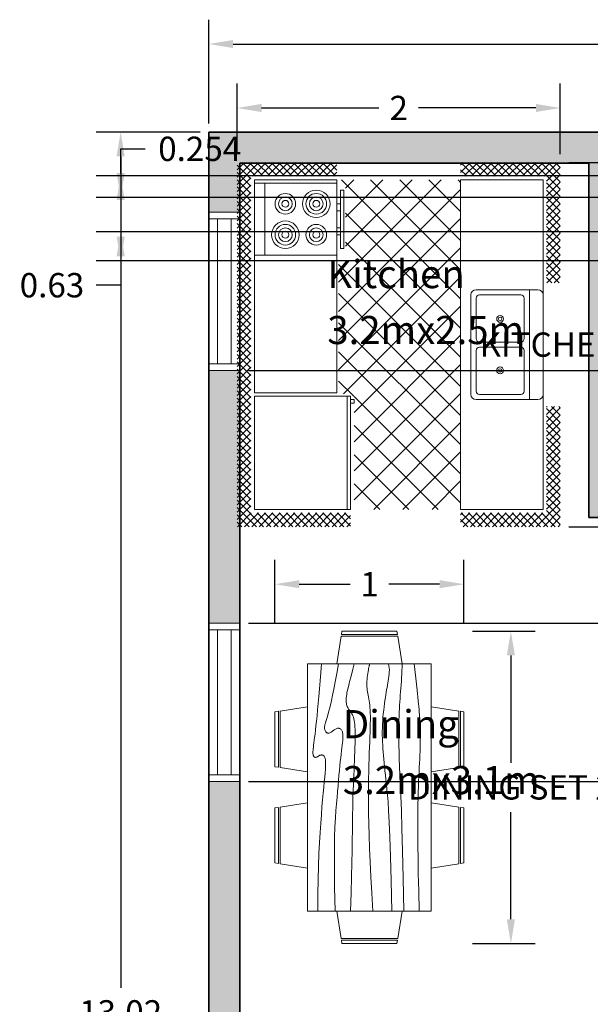
# Model space of a CAD drawing. Units: metres. Extents: x 35.2 to 46.4, y 446.1 to 460.8.
# Tile 5 of 6: x 36.2 to 40.4, y 453.5 to 460.8. Entities that reach past the tile are written whole.
import ezdxf

# ---------------------------------------------------------------- set-up
doc = ezdxf.new("R2010")
doc.units = ezdxf.units.M
for name, color, linetype, lineweight in [('A-ANNO-DIMS', 2, 'Continuous', 18), ('A-AREA-IDEN', 7, 'Continuous', 18), ('A-FLOR-FIXT', 9, 'Continuous', 18), ('A-GLAZ', 4, 'Continuous', 18), ('A-WALL', 7, 'Continuous', 35), ('A-WALL-PATT', 252, 'Continuous', 13), ('FURNITURE', 53, 'Continuous', 18)]:
    doc.layers.add(name, color=color, linetype=linetype, lineweight=lineweight)
doc.styles.get("Standard").update_dxf_attribs({"font": 'calibri.ttf'})
doc.dimstyles.get("Standard").update_dxf_attribs({"dimtxt": 0.18, "dimasz": 0.18, "dimexe": 0.18, "dimexo": 0.0625, "dimgap": 0.09, "dimtad": 0, "dimtih": 1, "dimtoh": 1, "dimdec": 4, "dimzin": 0, "dimdsep": 46, "dimtxsty": 'Standard', "dimcen": 0.09, "dimadec": 0, "dimazin": 0, "dimtfac": 1, "dimtdec": 4, "dimtofl": 0, "dimtmove": 0, "dimatfit": 3, "dimfxl": 1, "dimtolj": 1, "dimtzin": 0, "dimarcsym": 0})

# ---------------------------------------------------------------- blocks, each defined once
blk = doc.blocks.new('Dining Set - 36 x 72 in.')
for p, q in [((-22.2343, 26.00059), (-23.4847, 17.99762)), ((-22.2304, 26), (-5.7608, 26)), ((-22, 27.5), (-22.1562, 26.50042)), ((-5.8416, 26.5), (-22.1534, 26.5)), ((-22, 27.5), (-6, 27.5)), ((-5.8437, 26.49966), (-6, 27.5)), ((-4.5152, 17.99762), (-5.7655, 25.99926)), ((5.7657, 26.00059), (4.5153, 17.99762)), ((5.7696, 26), (22.2392, 26)), ((6, 27.5), (5.8438, 26.50042)), ((22.1584, 26.5), (5.8466, 26.5)), ((6, 27.5), (22, 27.5)), ((22.1563, 26.49966), (22, 27.5)), ((23.4848, 17.99762), (22.2345, 25.99926)), ((36, 18), (-36, 18)), ((-36, 18), (-36, -18)), ((36, -18), (36, 18)), ((-44.0006, 8.23428), (-35.9976, 9.48474)), ((44.0006, 8.23428), (35.9976, 9.48474)), ((-45.5, 8), (-44.5004, 8.15617)), ((-45.5, 8), (-45.5, -8)), ((-44.5, -8.15843), (-44.5, 8.15338)), ((-44, 8.23041), (-44, -8.23915)), ((44, 8.23041), (44, -8.23915)), ((44.5, -8.15843), (44.5, 8.15338)), ((45.5, 8), (44.5005, 8.15617)), ((45.5, 8), (45.5, -8)), ((-44.4997, -8.15631), (-45.5, -8)), ((-35.9976, -9.48476), (-43.9993, -8.2345)), ((35.9976, -9.48476), (43.9993, -8.2345)), ((44.4997, -8.15631), (45.5, -8)), ((-36, -18), (36, -18)), ((-22.2343, -26.0006), (-23.4847, -17.99762)), ((-4.5152, -17.99762), (-5.7655, -25.99928)), ((5.7657, -26.0006), (4.5153, -17.99762)), ((23.4848, -17.99762), (22.2345, -25.99928)), ((-22.2304, -26), (-5.7608, -26)), ((-22, -27.5), (-22.1562, -26.50044)), ((-5.8416, -26.5), (-22.1534, -26.5)), ((-22, -27.5), (-6, -27.5)), ((-5.8437, -26.49967), (-6, -27.5)), ((5.7696, -26), (22.2392, -26)), ((6, -27.5), (5.8438, -26.50044)), ((22.1584, -26.5), (5.8466, -26.5)), ((6, -27.5), (22, -27.5)), ((22.1563, -26.49967), (22, -27.5))]:
    blk.add_line(p, q)
for points in [[(-36, 15), (-31.1772, 14.97754), (-26.8079, 14.91406), (-22.8538, 14.81543), (-19.276, 14.6875), (-16.0362, 14.53613), (-13.0957, 14.36718), (-10.4159, 14.18652), (-7.9583, 14), (-5.6904, 13.81315), (-3.6035, 13.63021), (-1.6954, 13.45508), (0.0365, 13.29166), (1.5945, 13.14388), (2.9811, 13.01562), (4.1988, 12.9108), (5.25, 12.83333), (6.1393, 12.78613), (6.8802, 12.76823), (7.4883, 12.77767), (7.9792, 12.8125), (8.3685, 12.87077), (8.6719, 12.95052), (8.9049, 13.0498), (9.0833, 13.16666), (9.2205, 13.29899), (9.3216, 13.44401), (9.3895, 13.59879), (9.4271, 13.76041), (9.4373, 13.92594), (9.4232, 14.09245), (9.3875, 14.257), (9.3333, 14.41666), (9.2638, 14.56917), (9.1836, 14.71484), (9.0975, 14.85465), (9.0104, 14.98958), (8.9272, 15.1206), (8.8529, 15.2487), (8.7922, 15.37483), (8.75, 15.5), (8.7305, 15.62467), (8.7344, 15.74739), (8.7617, 15.86621), (8.8125, 15.97916), (8.8867, 16.08431), (8.9844, 16.17968), (9.1055, 16.26334), (9.25, 16.33333), (9.4189, 16.38802), (9.6172, 16.42708), (9.8506, 16.45052), (10.125, 16.45833), (10.4463, 16.45052), (10.8203, 16.42708), (11.2529, 16.38802), (11.75, 16.33333), (12.3184, 16.26318), (12.9694, 16.17838), (13.7151, 16.07991), (14.5677, 15.96875), (15.5395, 15.84586), (16.6426, 15.71224), (17.8893, 15.56884), (19.2917, 15.41666), (20.859, 15.25667), (22.5879, 15.08984), (24.4721, 14.91715), (26.5052, 14.73958), (28.6809, 14.5581), (30.9929, 14.3737), (33.4347, 14.18733), (36, 14)], [(-36, 10), (-28.9766, 10.14274), (-23.1725, 10.20442), (-18.4241, 10.19775), (-14.5677, 10.13541), (-11.4399, 10.03011), (-8.877, 9.89453), (-6.7154, 9.74137), (-4.7917, 9.58333), (-2.9698, 9.43082), (-1.2246, 9.28515), (0.4415, 9.14534), (2.026, 9.01041), (3.5266, 8.87939), (4.9408, 8.7513), (6.266, 8.62516), (7.5, 8.5), (8.6411, 8.37549), (9.6914, 8.2539), (10.6538, 8.13818), (11.5312, 8.03125), (12.3267, 7.93603), (13.043, 7.85547), (13.6831, 7.79248), (14.25, 7.75), (14.7471, 7.7303), (15.1797, 7.73307), (15.5537, 7.75732), (15.875, 7.80208), (16.1494, 7.86637), (16.3828, 7.94922), (16.5811, 8.04964), (16.75, 8.16666), (16.8944, 8.29915), (17.0143, 8.44531), (17.1089, 8.60319), (17.1771, 8.77083), (17.218, 8.94629), (17.2305, 9.1276), (17.2137, 9.31282), (17.1667, 9.5), (17.0895, 9.6875), (16.987, 9.875), (16.8649, 10.0625), (16.7292, 10.25), (16.5856, 10.4375), (16.4401, 10.625), (16.2985, 10.8125), (16.1667, 11), (16.05, 11.18733), (15.9518, 11.3737), (15.8752, 11.5581), (15.8229, 11.73958), (15.798, 11.91715), (15.8034, 12.08984), (15.842, 12.25667), (15.9167, 12.41666), (16.0295, 12.56836), (16.1784, 12.70833), (16.3605, 12.83268), (16.5729, 12.9375), (16.8127, 13.01888), (17.0768, 13.07291), (17.3625, 13.0957), (17.6667, 13.08333), (17.9894, 13.03312), (18.3418, 12.94726), (18.7382, 12.82918), (19.1927, 12.68229), (19.7195, 12.51001), (20.3327, 12.31575), (21.0465, 12.10294), (21.875, 11.875), (22.8357, 11.63354), (23.959, 11.37304), (25.2786, 11.08618), (26.8282, 10.76562), (28.6414, 10.40405), (30.752, 9.99414), (33.1936, 9.52856), (36, 9)], [(-36, 5.5), (-30.7157, 5.3348), (-26.069, 5.20963), (-21.9946, 5.11767), (-18.4271, 5.05208), (-15.3009, 5.00602), (-12.5508, 4.97265), (-10.1112, 4.94515), (-7.9167, 4.91666), (-5.909, 4.88167), (-4.0586, 4.83984), (-2.3429, 4.79215), (-0.7396, 4.73958), (0.7739, 4.6831), (2.22, 4.6237), (3.6213, 4.56233), (5, 4.5), (6.373, 4.43782), (7.7344, 4.3776), (9.0723, 4.32129), (10.375, 4.27083), (11.6309, 4.22819), (12.8281, 4.19531), (13.9551, 4.17415), (15, 4.16666), (15.954, 4.17448), (16.819, 4.19791), (17.6001, 4.23698), (18.3021, 4.29166), (18.9299, 4.36198), (19.4883, 4.44791), (19.9823, 4.54948), (20.4167, 4.66666), (20.7969, 4.79899), (21.1302, 4.94401), (21.4245, 5.09879), (21.6875, 5.26041), (21.9271, 5.42594), (22.1511, 5.59245), (22.3672, 5.757), (22.5834, 5.91666), (22.8065, 6.06868), (23.0404, 6.21093), (23.2879, 6.34147), (23.5521, 6.45833), (23.8358, 6.55957), (24.142, 6.64323), (24.4735, 6.70735), (24.8334, 6.75), (25.2235, 6.76969), (25.642, 6.76692), (26.0858, 6.74267), (26.5521, 6.69791), (27.0379, 6.63362), (27.5404, 6.55078), (28.0565, 6.45036), (28.5834, 6.33333), (29.1242, 6.19987), (29.7071, 6.04687), (30.3661, 5.87044), (31.1354, 5.66666), (32.0493, 5.43164), (33.142, 5.16146), (34.4475, 4.85221), (36, 4.5)], [(-36, -1), (-30.7915, -0.6591), (-26.0195, -0.38216), (-21.6519, -0.16284), (-17.6563, 0.00521), (-14.0005, 0.12833), (-10.6523, 0.21289), (-7.5796, 0.26522), (-4.75, 0.29166), (-2.134, 0.29793), (0.2878, 0.28711), (2.5317, 0.26163), (4.6146, 0.22396), (6.5529, 0.17651), (8.3633, 0.12174), (10.0623, 0.06209), (11.6667, 0), (13.1899, -0.06201), (14.6341, -0.1211), (15.9982, -0.17432), (17.2813, -0.21875), (18.4823, -0.25147), (19.6003, -0.26953), (20.6343, -0.27002), (21.5834, -0.25), (22.4481, -0.20768), (23.2357, -0.14584), (23.9549, -0.06836), (24.6146, 0.02083), (25.2235, 0.11784), (25.7904, 0.21875), (26.3241, 0.31966), (26.8334, 0.41666), (27.3265, 0.50618), (27.8099, 0.58593), (28.2894, 0.65397), (28.7709, 0.70833), (29.2601, 0.74707), (29.763, 0.76823), (30.2855, 0.76985), (30.8334, 0.75), (31.4088, 0.70784), (31.9994, 0.64713), (32.589, 0.57275), (33.1615, 0.48958), (33.7008, 0.4025), (34.1908, 0.3164), (34.6153, 0.23616), (34.9584, 0.16666), (35.2099, 0.11165), (35.3848, 0.07031), (35.504, 0.04069), (35.5886, 0.02083), (35.6594, 0.00879), (35.7377, 0.0026), (35.8442, 0.00032), (36, 0)], [(-36, -6.5), (-27.1843, -6.31267), (-20.084, -6.1263), (-14.469, -5.9419), (-10.1094, -5.76042), (-6.7752, -5.58285), (-4.2363, -5.41016), (-2.2629, -5.24333), (-0.625, -5.08334), (0.8708, -4.93099), (2.2715, -4.78646), (3.5872, -4.64974), (4.8281, -4.52084), (6.0046, -4.39974), (7.127, -4.28646), (8.2053, -4.18099), (9.25, -4.08334), (10.2705, -3.99382), (11.2734, -3.91407), (12.2647, -3.84603), (13.25, -3.79167), (14.2354, -3.75293), (15.2266, -3.73177), (16.2295, -3.73015), (17.25, -3.75), (18.2912, -3.79248), (19.3451, -3.85547), (20.4009, -3.93604), (21.4479, -4.03125), (22.4754, -4.13819), (23.4727, -4.25391), (24.4289, -4.37549), (25.3334, -4.5), (26.1785, -4.62492), (26.9694, -4.74935), (27.7145, -4.87281), (28.4219, -4.99479), (29.1, -5.11483), (29.7572, -5.23242), (30.4016, -5.34709), (31.0417, -5.45834), (31.6837, -5.56437), (32.3262, -5.65821), (32.9658, -5.73153), (33.599, -5.77604), (34.2224, -5.78345), (34.8327, -5.74545), (35.4264, -5.65373), (36, -5.5)], [(-36, -10), (-26.4022, -9.81299), (-18.4675, -9.62891), (-11.9839, -9.45069), (-6.7396, -9.28125), (-2.5226, -9.12354), (0.8789, -8.98047), (3.6769, -8.85498), (6.0833, -8.75), (8.2767, -8.66765), (10.3021, -8.60677), (12.1712, -8.56543), (13.8958, -8.54167), (15.4876, -8.53353), (16.9583, -8.53907), (18.3197, -8.55632), (19.5834, -8.58334), (20.7616, -8.61841), (21.8685, -8.66081), (22.9188, -8.71004), (23.9271, -8.76563), (24.9081, -8.82707), (25.8763, -8.89388), (26.8465, -8.96558), (27.8334, -9.04167), (28.8474, -9.12118), (29.8828, -9.20117), (30.93, -9.27824), (31.9792, -9.34896), (33.0205, -9.40991), (34.0443, -9.45768), (35.0407, -9.48885), (36, -9.5)], [(-36, -14.5), (-30.0881, -14.33513), (-25.0332, -14.21224), (-20.7312, -14.12647), (-17.0781, -14.07292), (-13.97, -14.04671), (-11.3027, -14.04297), (-8.9724, -14.05681), (-6.875, -14.08334), (-4.9224, -14.11833), (-3.0905, -14.16016), (-1.3709, -14.20785), (0.2448, -14.26042), (1.7647, -14.3169), (3.1973, -14.3763), (4.5507, -14.43767), (5.8333, -14.5), (7.0554, -14.5621), (8.235, -14.62175), (9.3922, -14.67652), (10.5469, -14.72396), (11.7192, -14.76164), (12.929, -14.78711), (14.1965, -14.79794), (15.5417, -14.79167), (16.9933, -14.76424), (18.6152, -14.70508), (20.4804, -14.60197), (22.6615, -14.44271), (25.2312, -14.21509), (28.2624, -13.9069), (31.8277, -13.50594), (36, -13)]]:
    blk.add_lwpolyline(points)
blk = doc.blocks.new('Kitchen Layout - 7 x 8 ft')
for p, q in [((-5, 81.32), (2.68, 89)), ((-5, 83.44), (0.56, 89)), ((-5, 85.56), (-1.56, 89)), ((-5, 87.68), (-3.68, 89)), ((-1, 84.97), (-5, 88.97)), ((1.09, 85), (-2.91, 89)), ((3.21, 85), (-0.79, 89)), ((0.81, 85), (4.81, 89)), ((5.34, 85), (1.34, 89)), ((2.93, 85), (6.93, 89)), ((7.46, 85), (3.46, 89)), ((5.05, 85), (9.05, 89)), ((9.58, 85), (5.58, 89)), ((7.17, 85), (11.17, 89)), ((11.7, 85), (7.7, 89)), ((9.29, 85), (13.29, 89)), ((13.82, 85), (9.82, 89)), ((11.41, 85), (15.41, 89)), ((15.94, 85), (11.94, 89)), ((13.53, 85), (17.53, 89)), ((18.06, 85), (14.06, 89)), ((15.65, 85), (19.65, 89)), ((20.18, 85), (16.18, 89)), ((17.78, 85), (21.78, 89)), ((22.31, 85), (18.31, 89)), ((19.9, 85), (23.9, 89)), ((24.43, 85), (20.43, 89)), ((22.02, 85), (26.02, 89)), ((26.55, 85), (22.55, 89)), ((24.14, 85), (28.14, 89)), ((28.67, 85), (24.67, 89)), ((26.26, 85), (30.26, 89)), ((30.79, 85), (26.79, 89)), ((28.38, 85), (32.38, 89)), ((32.91, 85), (28.91, 89)), ((30.5, 85), (34.5, 89)), ((35.03, 85), (31.03, 89)), ((32.63, 85), (36.63, 89)), ((37.16, 85), (33.16, 89)), ((34.75, 85), (38.75, 89)), ((39.28, 85), (35.28, 89)), ((36.87, 85), (40.87, 89)), ((41.4, 85), (37.4, 89)), ((38.99, 85), (42.99, 89)), ((43.52, 85), (39.52, 89)), ((41.11, 85), (45.11, 89)), ((45.64, 85), (41.64, 89)), ((43.23, 85), (47.23, 89)), ((47.76, 85), (43.76, 89)), ((45.35, 85), (49.35, 89)), ((49.88, 85), (45.88, 89)), ((47.47, 85), (51.47, 89)), ((52, 85), (48, 89)), ((49.6, 85), (53.6, 89)), ((54.13, 85), (50.13, 89)), ((51.72, 85), (55.72, 89)), ((56.25, 85), (52.25, 89)), ((53.84, 85), (57.84, 89)), ((58.37, 85), (54.37, 89)), ((55.96, 85), (59.96, 89)), ((60.49, 85), (56.49, 89)), ((58.08, 85), (62.08, 89)), ((62.61, 85), (58.61, 89)), ((60.2, 85), (64.2, 89)), ((64.73, 85), (60.73, 89)), ((62.32, 85), (66.32, 89)), ((66.85, 85), (62.85, 89)), ((64.45, 85), (68.45, 89)), ((68.97, 85), (64.97, 89)), ((66.57, 85), (70.57, 89)), ((71.1, 85), (67.1, 89)), ((68.69, 85), (72.69, 89)), ((73.22, 85), (69.22, 89)), ((70.81, 85), (74.81, 89)), ((75.34, 85), (71.34, 89)), ((72.93, 85), (76.93, 89)), ((77.46, 85), (73.46, 89)), ((75.05, 85), (79.05, 89)), ((79.58, 85), (75.58, 89)), ((77.17, 85), (81.17, 89)), ((81.7, 85), (77.7, 89)), ((79.29, 85), (83.29, 89)), ((83.82, 85), (79.82, 89)), ((81.42, 85), (85.42, 89)), ((85.95, 85), (81.95, 89)), ((83.54, 85), (87.54, 89)), ((88.07, 85), (84.07, 89)), ((85.66, 85), (89.66, 89)), ((90.19, 85), (86.19, 89)), ((87.78, 85), (91.78, 89)), ((92.31, 85), (88.31, 89)), ((89.9, 85), (93.9, 89)), ((94.43, 85), (90.43, 89)), ((92.02, 85), (96.02, 89)), ((96.55, 85), (92.55, 89)), ((94.14, 85), (98.14, 89)), ((101, 82.67), (94.67, 89)), ((96.27, 85), (100.27, 89)), ((101, 84.79), (96.79, 89)), ((101, 86.92), (98.92, 89)), ((-1, 82.85), (-5, 86.85)), ((97, 83.61), (101, 87.61)), ((-1, 80.73), (-5, 84.73)), ((-5, 79.19), (-1, 83.19)), ((34, 84), (96, 84)), ((34, 60), (34, 84)), ((96, 84), (96, 60)), ((97, 81.49), (101, 85.49)), ((101, 80.55), (97, 84.55)), ((97, 79.37), (101, 83.37)), ((-1, 78.61), (-5, 82.61)), ((-5, 77.07), (-1, 81.07)), ((-1, 76.49), (-5, 80.49)), ((74, 81), (95, 81)), ((101, 78.43), (97, 82.43)), ((97, 77.25), (101, 81.25)), ((101, 76.31), (97, 80.31)), ((-5, 74.95), (-1, 78.95)), ((-1, 74.36), (-5, 78.36)), ((97, 75.13), (101, 79.13)), ((101, 74.19), (97, 78.19)), ((-5, 72.83), (-1, 76.83)), ((-1, 72.24), (-5, 76.24)), ((-5, 70.71), (-1, 74.71)), ((97, 73.01), (101, 77.01)), ((101, 72.07), (97, 76.07)), ((97, 70.89), (101, 74.89)), ((-1, 70.12), (-5, 74.12)), ((-5, 68.59), (-1, 72.59)), ((-1, 68), (-5, 72)), ((101, 69.95), (97, 73.95)), ((97, 68.76), (101, 72.76)), ((101, 67.82), (97, 71.82)), ((-5, 66.47), (-1, 70.47)), ((-1, 65.88), (-5, 69.88)), ((97, 66.64), (101, 70.64)), ((101, 65.7), (97, 69.7)), ((-5, 64.35), (-1, 68.35)), ((-1, 63.76), (-5, 67.76)), ((-5, 62.22), (-1, 66.22)), ((97, 64.52), (101, 68.52)), ((101, 63.58), (97, 67.58)), ((97, 62.4), (101, 66.4)), ((-1, 61.64), (-5, 65.64)), ((-5, 60.1), (-1, 64.1)), ((-1, 59.52), (-5, 63.52)), ((101, 61.46), (97, 65.46)), ((97, 60.28), (101, 64.28)), ((100.34, 60), (97, 63.34)), ((-5, 57.98), (-1, 61.98)), ((-1, 57.39), (-5, 61.39)), ((98.22, 60), (97, 61.22)), ((98.84, 60), (101, 62.16)), ((-1.73, 56), (-5, 59.27)), ((-4.86, 56), (-1, 59.86)), ((-2.74, 56), (-1, 57.74)), ((10.4, 24), (45.9, 59.5)), ((18.88, 24), (54.38, 59.5)), ((27.37, 24), (62.87, 59.5)), ((33.03, 55.11), (37.41, 59.5)), ((67.71, 24), (33.68, 58.04)), ((96, 60), (34, 60)), ((35.85, 24), (71.35, 59.5)), ((76.2, 24), (40.7, 59.5)), ((44.34, 24), (77.84, 57.5)), ((84.68, 24), (49.18, 59.5)), ((52.82, 24), (86.32, 57.5)), ((93.17, 24), (57.67, 59.5)), ((61.31, 24), (96, 58.69)), ((96, 29.65), (66.15, 59.5)), ((96, 38.14), (76.64, 57.5)), ((80, 60), (80, 59)), ((82, 59), (82, 60)), ((96, 46.63), (85.13, 57.5)), ((87, 59), (87, 60)), ((89, 60), (89, 59)), ((96, 55.11), (93.57, 57.54)), ((100.96, 60), (101, 60.04)), ((-3.85, 56), (-5, 57.15)), ((0, 57), (33, 57)), ((0, 30.57), (24.43, 55)), ((0, 39.06), (15.94, 55)), ((0, 47.54), (7.46, 55)), ((1.91, 24), (32.91, 55)), ((33.77, 24), (2.77, 55)), ((42.26, 24), (11.26, 55)), ((50.74, 24), (19.74, 55)), ((59.23, 24), (28.23, 55)), ((31, 55), (31, 56)), ((32, 55), (31, 55)), ((32, 56), (32, 55)), ((25.29, 24), (0, 49.29)), ((69.79, 24), (96, 50.21)), ((16.8, 24), (0, 40.8)), ((78.28, 24), (96, 41.72)), ((8.32, 24), (0, 32.32)), ((86.76, 24), (96, 33.24)), ((-5, 21.92), (-2.92, 24)), ((-5, 19.8), (-1, 23.8)), ((-1, 19.21), (-5, 23.21)), ((-1, 21.33), (-3.67, 24)), ((-1, 23.45), (-1.55, 24)), ((0, 24), (96, 24)), ((0, 0), (0, 24)), ((95.25, 24), (96, 24.75)), ((96, 24), (96, 0)), ((97, 22.1), (98.9, 24)), ((97, 19.97), (101, 23.97)), ((101, 19.03), (97, 23.03)), ((101, 21.16), (98.16, 24)), ((101, 23.28), (100.28, 24)), ((-5, 17.68), (-1, 21.68)), ((-1, 17.09), (-5, 21.09)), ((97, 17.85), (101, 21.85)), ((101, 16.91), (97, 20.91)), ((-5, 15.55), (-1, 19.55)), ((-1, 14.97), (-5, 18.97)), ((-5, 13.43), (-1, 17.43)), ((47.25, 6.5), (47.25, 18.5)), ((48.75, 18.5), (48.75, 6.5)), ((97, 15.73), (101, 19.73)), ((101, 14.79), (97, 18.79)), ((97, 13.61), (101, 17.61)), ((-1, 12.85), (-5, 16.85)), ((-5, 11.31), (-1, 15.31)), ((-1, 10.73), (-5, 14.73)), ((101, 12.67), (97, 16.67)), ((97, 11.49), (101, 15.49)), ((101, 10.55), (97, 14.55)), ((-5, 9.19), (-1, 13.19)), ((-1, 8.6), (-5, 12.6)), ((97, 9.37), (101, 13.37)), ((101, 8.43), (97, 12.43)), ((-5, 7.07), (-1, 11.07)), ((-1, 6.48), (-5, 10.48)), ((-5, 4.95), (-1, 8.95)), ((97, 7.25), (101, 11.25)), ((101, 6.31), (97, 10.31)), ((97, 5.12), (101, 9.12)), ((-1, 4.36), (-5, 8.36)), ((-5, 2.83), (-1, 6.83)), ((-1, 2.24), (-5, 6.24)), ((101, 4.18), (97, 8.18)), ((97, 3), (101, 7)), ((101, 2.06), (97, 6.06)), ((-5, 0.71), (-1, 4.71)), ((-1, 0.12), (-5, 4.12)), ((64, 4), (32, 4)), ((97, 0.88), (101, 4.88)), ((101, -0.06), (97, 3.94)), ((-5, -1.42), (-1, 2.58)), ((2, -5), (-5, 2)), ((-5, -3.54), (-1, 0.46)), ((96, 0), (0, 0)), ((93.24, -5), (101, 2.76)), ((95.36, -5), (101, 0.64)), ((101, -2.18), (97, 1.82)), ((-0.12, -5), (-5, -0.12)), ((-2.25, -5), (-5, -2.25)), ((-4.34, -5), (-0.34, -1)), ((-2.22, -5), (1.78, -1)), ((-0.1, -5), (3.9, -1)), ((4.12, -5), (0.12, -1)), ((2.02, -5), (6.02, -1)), ((6.24, -5), (2.24, -1)), ((4.14, -5), (8.14, -1)), ((8.36, -5), (4.36, -1)), ((6.27, -5), (10.27, -1)), ((10.48, -5), (6.48, -1)), ((8.39, -5), (12.39, -1)), ((12.6, -5), (8.6, -1)), ((10.51, -5), (14.51, -1)), ((14.73, -5), (10.73, -1)), ((12.63, -5), (16.63, -1)), ((16.85, -5), (12.85, -1)), ((14.75, -5), (18.75, -1)), ((18.97, -5), (14.97, -1)), ((16.87, -5), (20.87, -1)), ((21.09, -5), (17.09, -1)), ((18.99, -5), (22.99, -1)), ((23.21, -5), (19.21, -1)), ((21.11, -5), (25.11, -1)), ((25.33, -5), (21.33, -1)), ((23.24, -5), (27.24, -1)), ((27.45, -5), (23.45, -1)), ((25.36, -5), (29.36, -1)), ((29.57, -5), (25.57, -1)), ((27.48, -5), (30, -2.48)), ((30, -3.3), (27.7, -1)), ((30, -1.18), (29.82, -1)), ((66, -2.54), (67.54, -1)), ((66, -4.66), (69.66, -1)), ((69.88, -5), (66, -1.12)), ((67.78, -5), (71.78, -1)), ((72, -5), (68, -1)), ((69.9, -5), (73.9, -1)), ((74.12, -5), (70.12, -1)), ((72.03, -5), (76.03, -1)), ((76.24, -5), (72.24, -1)), ((74.15, -5), (78.15, -1)), ((78.36, -5), (74.36, -1)), ((76.27, -5), (80.27, -1)), ((80.49, -5), (76.49, -1)), ((78.39, -5), (82.39, -1)), ((82.61, -5), (78.61, -1)), ((80.51, -5), (84.51, -1)), ((84.73, -5), (80.73, -1)), ((82.63, -5), (86.63, -1)), ((86.85, -5), (82.85, -1)), ((84.75, -5), (88.75, -1)), ((88.97, -5), (84.97, -1)), ((86.88, -5), (90.88, -1)), ((91.09, -5), (87.09, -1)), ((89, -5), (93, -1)), ((93.21, -5), (89.21, -1)), ((91.12, -5), (95.12, -1)), ((95.34, -5), (91.34, -1)), ((97.46, -5), (93.46, -1)), ((99.58, -5), (95.58, -1)), ((101, -4.3), (97, -0.3)), ((97.48, -5), (101, -1.48)), ((-4.37, -5), (-5, -4.37)), ((29.6, -5), (30, -4.6)), ((67.76, -5), (66, -3.24)), ((99.6, -5), (101, -3.6))]:
    blk.add_line(p, q)
for points in [[(0, 56), (0, 84), (33, 84), (33, 56)], [(74, 60), (74, 84), (95, 84), (95, 60)], [(76, 58), (76, 59), (93, 59), (93, 58)]]:
    blk.add_lwpolyline(points, close=True)
for points in [[(33.5, 21), (62.5, 21)], [(32, 1.5), (32, 19.5)], [(33.5, 6.5), (33.5, 18.5)], [(34.5, 19.5), (46.25, 19.5)], [(49.75, 19.5), (61.5, 19.5)], [(62.5, 18.5), (62.5, 6.5)], [(64, 19.5), (64, 1.5)], [(46.25, 5.5), (34.5, 5.5)], [(61.5, 5.5), (49.75, 5.5)], [(62.5, 0), (33.5, 0)]]:
    blk.add_lwpolyline(points)
for centre, radius in [((80, 75), 4), ((80, 75), 3), ((89, 75), 3), ((80, 75), 2), ((80, 75), 1), ((89, 75), 2), ((89, 75), 1), ((80, 66), 3), ((89, 66), 4), ((89, 66), 3), ((80, 66), 2), ((80, 66), 1), ((89, 66), 2), ((89, 66), 1), ((40.5, 12.5), 1), ((40.5, 12.5), 0.5), ((55.5, 12.5), 1), ((55.5, 12.5), 0.5)]:
    blk.add_circle(centre, radius)
for centre, radius, start, end in [((33.5, 19.5), 1.5, 90, 180), ((62.5, 19.5), 1.5, 0, 90), ((34.5, 18.5), 1, 90, 180), ((46.25, 18.5), 1, 0, 90), ((49.75, 18.5), 1, 90, 180), ((61.5, 18.5), 1, 0, 90), ((34.5, 6.5), 1, 180, 270), ((46.25, 6.5), 1, 270, 0), ((49.75, 6.5), 1, 180, 270), ((61.5, 6.5), 1, 270, 0), ((33.5, 1.5), 1.5, 180, 270), ((62.5, 1.5), 1.5, 270, 0)]:
    blk.add_arc(centre, radius, start, end)
blk = doc.blocks.new('WIN-1172')
for p, q in [((0, 1.1716), (0.23, 1.1716)), ((0, 1.1716), (0, 0)), ((0.23, 1.1716), (0.23, 0)), ((0, 1.1216), (0.23, 1.1216)), ((0.065, 1.1216), (0.065, 0.05)), ((0.165, 1.1216), (0.165, 0.05)), ((0.23, 0.05), (0, 0.05)), ((0.23, 0), (0, 0))]:
    blk.add_line(p, q)
blk = doc.blocks.new('*D139')
at = {"layer": 'A-ANNO-DIMS', "color": 0, "lineweight": -2, "transparency": 16777216}
for p, q in [((39.5553, 456.2345), (40.0195, 456.2345)), ((39.8395, 456.0545), (39.8395, 455.261)), ((39.8395, 454.1031), (39.8395, 454.8966)), ((39.5553, 453.9231), (40.0195, 453.9231))]:
    blk.add_line(p, q, dxfattribs=at)
at = {"layer": 'A-ANNO-DIMS', "color": 0, "transparency": 16777216}
for points in [[(39.8095, 456.0545), (39.8695, 456.0545), (39.8395, 456.2345)], [(39.8095, 454.1031), (39.8695, 454.1031), (39.8395, 453.9231)]]:
    blk.add_solid(points, dxfattribs=at)
at = {"layer": 'Defpoints', "color": 0, "transparency": 16777216}
for p in [(39.4928, 456.2345), (39.8395, 456.2345), (39.4928, 453.9231)]:
    blk.add_point(p, dxfattribs=at)
at = {"layer": 'A-ANNO-DIMS', "color": 0, "transparency": 16777216, "insert": (39.8395, 455.0788), "char_height": 0.18, "attachment_point": 5}
blk.add_mtext('\\A1;DINING SET 2', dxfattribs=at)
blk = doc.blocks.new('*D140')
at = {"layer": 'A-ANNO-DIMS', "color": 0, "lineweight": -2, "transparency": 16777216}
for p, q in [((38.0958, 456.297), (38.0958, 456.7612)), ((39.4928, 456.297), (39.4928, 456.7612)), ((38.2758, 456.5812), (38.6522, 456.5812)), ((39.3128, 456.5812), (38.9364, 456.5812))]:
    blk.add_line(p, q, dxfattribs=at)
at = {"layer": 'A-ANNO-DIMS', "color": 0, "transparency": 16777216}
for points in [[(38.2758, 456.6112), (38.2758, 456.5512), (38.0958, 456.5812)], [(39.3128, 456.6112), (39.3128, 456.5512), (39.4928, 456.5812)]]:
    blk.add_solid(points, dxfattribs=at)
at = {"layer": 'Defpoints', "color": 0, "transparency": 16777216}
for p in [(38.0958, 456.5812), (38.0958, 456.2345), (39.4928, 456.2345)]:
    blk.add_point(p, dxfattribs=at)
at = {"layer": 'A-ANNO-DIMS', "color": 0, "transparency": 16777216, "insert": (38.7943, 456.5812), "char_height": 0.18, "attachment_point": 5}
blk.add_mtext('\\A1;1', dxfattribs=at)
blk = doc.blocks.new('*D145')
at = {"layer": 'A-ANNO-DIMS', "color": 0, "lineweight": -2, "transparency": 16777216}
for p, q in [((40.2671, 459.6992), (40.7885, 459.6992)), ((40.6085, 459.5192), (40.6085, 458.5353)), ((40.6085, 457.1868), (40.6085, 458.1708)), ((40.2671, 457.0068), (40.7885, 457.0068))]:
    blk.add_line(p, q, dxfattribs=at)
at = {"layer": 'A-ANNO-DIMS', "color": 0, "transparency": 16777216}
for points in [[(40.5785, 459.5192), (40.6385, 459.5192), (40.6085, 459.6992)], [(40.5785, 457.1868), (40.6385, 457.1868), (40.6085, 457.0068)]]:
    blk.add_solid(points, dxfattribs=at)
at = {"layer": 'Defpoints', "color": 0, "transparency": 16777216}
for p in [(40.2046, 459.6992), (40.6085, 459.6992), (40.2046, 457.0068)]:
    blk.add_point(p, dxfattribs=at)
at = {"layer": 'A-ANNO-DIMS', "color": 0, "transparency": 16777216, "insert": (40.6085, 458.353), "char_height": 0.18, "attachment_point": 5}
blk.add_mtext('\\A1;KITCHEN UNITS 3', dxfattribs=at)
blk = doc.blocks.new('*D146')
at = {"layer": 'A-ANNO-DIMS', "color": 0, "lineweight": -2, "transparency": 16777216}
for p, q in [((37.817, 459.7617), (37.817, 460.2831)), ((40.2046, 459.7617), (40.2046, 460.2831)), ((37.997, 460.1031), (38.8647, 460.1031)), ((40.0246, 460.1031), (39.1569, 460.1031))]:
    blk.add_line(p, q, dxfattribs=at)
at = {"layer": 'A-ANNO-DIMS', "color": 0, "transparency": 16777216}
for points in [[(37.997, 460.1331), (37.997, 460.0731), (37.817, 460.1031)], [(40.0246, 460.1331), (40.0246, 460.0731), (40.2046, 460.1031)]]:
    blk.add_solid(points, dxfattribs=at)
at = {"layer": 'Defpoints', "color": 0, "transparency": 16777216}
for p in [(37.817, 460.1031), (37.817, 459.6992), (40.2046, 459.6992)]:
    blk.add_point(p, dxfattribs=at)
at = {"layer": 'A-ANNO-DIMS', "color": 0, "transparency": 16777216, "insert": (39.0108, 460.1031), "char_height": 0.18, "attachment_point": 5}
blk.add_mtext('\\A1;2', dxfattribs=at)
blk = doc.blocks.new('*D151')
at = {"layer": 'A-ANNO-DIMS', "color": 0, "lineweight": -2, "transparency": 16777216}
for p, q in [((37.6066, 459.9873), (37.6066, 460.756)), ((44.9866, 459.9873), (44.9866, 460.756)), ((37.7866, 460.576), (40.9679, 460.576)), ((44.8066, 460.576), (41.6253, 460.576))]:
    blk.add_line(p, q, dxfattribs=at)
at = {"layer": 'A-ANNO-DIMS', "color": 0, "transparency": 16777216}
for points in [[(37.7866, 460.606), (37.7866, 460.546), (37.6066, 460.576)], [(44.8066, 460.606), (44.8066, 460.546), (44.9866, 460.576)]]:
    blk.add_solid(points, dxfattribs=at)
at = {"layer": 'Defpoints', "color": 0, "transparency": 16777216}
for p in [(44.9866, 460.576), (37.6066, 459.9248), (44.9866, 459.9248)]:
    blk.add_point(p, dxfattribs=at)
at = {"layer": 'A-ANNO-DIMS', "color": 0, "transparency": 16777216, "insert": (41.2966, 460.576), "char_height": 0.18, "attachment_point": 5}
blk.add_mtext('\\A1;7.38', dxfattribs=at)
blk = doc.blocks.new('*D152')
at = {"layer": 'A-ANNO-DIMS', "color": 0, "lineweight": -2, "transparency": 16777216}
for p, q in [((37.5441, 459.9248), (36.7754, 459.9248)), ((36.9554, 459.7448), (36.9554, 453.597)), ((36.9554, 447.0848), (36.9554, 453.2326)), ((37.5441, 446.9048), (36.7754, 446.9048))]:
    blk.add_line(p, q, dxfattribs=at)
at = {"layer": 'A-ANNO-DIMS', "color": 0, "transparency": 16777216}
for points in [[(36.9254, 459.7448), (36.9854, 459.7448), (36.9554, 459.9248)], [(36.9254, 447.0848), (36.9854, 447.0848), (36.9554, 446.9048)]]:
    blk.add_solid(points, dxfattribs=at)
at = {"layer": 'Defpoints', "color": 0, "transparency": 16777216}
for p in [(36.9554, 459.9248), (37.6066, 459.9248), (37.6066, 446.9048)]:
    blk.add_point(p, dxfattribs=at)
at = {"layer": 'A-ANNO-DIMS', "color": 0, "transparency": 16777216, "insert": (36.9554, 453.4148), "char_height": 0.18, "attachment_point": 5}
blk.add_mtext('\\A1;13.02', dxfattribs=at)
blk = doc.blocks.new('*D156')
at = {"layer": 'A-ANNO-DIMS', "color": 0, "lineweight": -2, "transparency": 16777216}
for p, q in [((37.8991, 455.122), (45.8178, 455.122)), ((45.6378, 454.942), (45.6378, 454.1543)), ((45.6378, 453.0022), (45.6378, 453.7898)), ((37.8991, 452.8222), (45.8178, 452.8222))]:
    blk.add_line(p, q, dxfattribs=at)
at = {"layer": 'A-ANNO-DIMS', "color": 0, "transparency": 16777216}
for points in [[(45.6078, 454.942), (45.6678, 454.942), (45.6378, 455.122)], [(45.6078, 453.0022), (45.6678, 453.0022), (45.6378, 452.8222)]]:
    blk.add_solid(points, dxfattribs=at)
at = {"layer": 'Defpoints', "color": 0, "transparency": 16777216}
for p in [(37.8366, 455.122), (45.6378, 455.122), (37.8366, 452.8222)]:
    blk.add_point(p, dxfattribs=at)
at = {"layer": 'A-ANNO-DIMS', "color": 0, "transparency": 16777216, "insert": (45.6378, 453.9721), "char_height": 0.18, "attachment_point": 5}
blk.add_mtext('\\A1;2.3', dxfattribs=at)
blk = doc.blocks.new('*D157')
at = {"layer": 'A-ANNO-DIMS', "color": 0, "lineweight": -2, "transparency": 16777216}
for p, q in [((37.8991, 456.2935), (45.8178, 456.2935)), ((45.6378, 456.1135), (45.6378, 455.8886)), ((45.6378, 455.302), (45.6378, 455.5269)), ((37.8991, 455.122), (45.8178, 455.122))]:
    blk.add_line(p, q, dxfattribs=at)
at = {"layer": 'A-ANNO-DIMS', "color": 0, "transparency": 16777216}
for points in [[(45.6078, 456.1135), (45.6678, 456.1135), (45.6378, 456.2935)], [(45.6078, 455.302), (45.6678, 455.302), (45.6378, 455.122)]]:
    blk.add_solid(points, dxfattribs=at)
at = {"layer": 'Defpoints', "color": 0, "transparency": 16777216}
for p in [(37.8366, 456.2935), (45.6378, 456.2935), (37.8366, 455.122)]:
    blk.add_point(p, dxfattribs=at)
at = {"layer": 'A-ANNO-DIMS', "color": 0, "transparency": 16777216, "insert": (45.6378, 455.7077), "char_height": 0.18, "attachment_point": 5}
blk.add_mtext('\\A1;1.17', dxfattribs=at)
blk = doc.blocks.new('*D158')
at = {"layer": 'A-ANNO-DIMS', "color": 0, "lineweight": -2, "transparency": 16777216}
for p, q in [((37.8991, 458.1617), (45.8178, 458.1617)), ((45.6378, 457.9817), (45.6378, 457.4098)), ((45.6378, 456.4735), (45.6378, 457.0454)), ((37.8991, 456.2935), (45.8178, 456.2935))]:
    blk.add_line(p, q, dxfattribs=at)
at = {"layer": 'A-ANNO-DIMS', "color": 0, "transparency": 16777216}
for points in [[(45.6078, 457.9817), (45.6678, 457.9817), (45.6378, 458.1617)], [(45.6078, 456.4735), (45.6678, 456.4735), (45.6378, 456.2935)]]:
    blk.add_solid(points, dxfattribs=at)
at = {"layer": 'Defpoints', "color": 0, "transparency": 16777216}
for p in [(37.8366, 458.1617), (45.6378, 458.1617), (37.8366, 456.2935)]:
    blk.add_point(p, dxfattribs=at)
at = {"layer": 'A-ANNO-DIMS', "color": 0, "transparency": 16777216, "insert": (45.6378, 457.2276), "char_height": 0.18, "attachment_point": 5}
blk.add_mtext('\\A1;1.87', dxfattribs=at)
blk = doc.blocks.new('*D167')
at = {"layer": 'A-ANNO-DIMS', "color": 0, "lineweight": -2, "transparency": 16777216}
for p, q in [((37.8366, 459.6323), (37.8366, 446.0736)), ((40.8069, 459.6323), (40.8069, 446.0736)), ((38.0166, 446.2536), (38.9948, 446.2536)), ((40.6269, 446.2536), (39.6486, 446.2536))]:
    blk.add_line(p, q, dxfattribs=at)
at = {"layer": 'A-ANNO-DIMS', "color": 0, "transparency": 16777216}
for points in [[(38.0166, 446.2836), (38.0166, 446.2236), (37.8366, 446.2536)], [(40.6269, 446.2836), (40.6269, 446.2236), (40.8069, 446.2536)]]:
    blk.add_solid(points, dxfattribs=at)
at = {"layer": 'Defpoints', "color": 0, "transparency": 16777216}
for p in [(37.8366, 459.6948), (40.8069, 459.6948), (40.8069, 446.2536)]:
    blk.add_point(p, dxfattribs=at)
at = {"layer": 'A-ANNO-DIMS', "color": 0, "transparency": 16777216, "insert": (39.3217, 446.2536), "char_height": 0.18, "attachment_point": 5}
blk.add_mtext('\\A1;2.97', dxfattribs=at)
blk = doc.blocks.new('*D169')
at = {"layer": 'A-ANNO-DIMS', "color": 0, "lineweight": -2, "transparency": 16777216}
for p, q in [((40.536595, 457.132279), (40.536595, 446.073579)), ((41.656595, 457.132279), (41.656595, 446.073579)), ((40.356595, 446.253579), (40.176595, 446.253579)), ((41.836595, 446.253579), (42.016595, 446.253579))]:
    blk.add_line(p, q, dxfattribs=at)
at = {"layer": 'A-ANNO-DIMS', "color": 0, "transparency": 16777216}
for points in [[(40.356595, 446.283579), (40.356595, 446.223579), (40.536595, 446.253579)], [(41.836595, 446.283579), (41.836595, 446.223579), (41.656595, 446.253579)]]:
    blk.add_solid(points, dxfattribs=at)
at = {"layer": 'Defpoints', "color": 0, "transparency": 16777216}
for p in [(40.536595, 457.194779), (41.656595, 457.194779), (41.656595, 446.253579)]:
    blk.add_point(p, dxfattribs=at)
at = {"layer": 'A-ANNO-DIMS', "color": 0, "transparency": 16777216, "insert": (41.096595, 446.253579), "char_height": 0.18, "attachment_point": 5}
blk.add_mtext('\\A1;1.12', dxfattribs=at)
blk = doc.blocks.new('*D177')
at = {"layer": 'A-ANNO-DIMS', "color": 0, "lineweight": -2, "transparency": 16777216}
for p, q in [((36.9554, 459.6211), (36.9554, 459.8011)), ((36.9554, 459.8011), (37.1354, 459.8011)), ((43.6711, 459.4411), (36.7754, 459.4411)), ((43.6711, 459.1871), (36.7754, 459.1871)), ((36.9554, 459.0071), (36.9554, 458.8271))]:
    blk.add_line(p, q, dxfattribs=at)
at = {"layer": 'A-ANNO-DIMS', "color": 0, "transparency": 16777216}
for points in [[(36.9254, 459.6211), (36.9854, 459.6211), (36.9554, 459.4411)], [(36.9254, 459.0071), (36.9854, 459.0071), (36.9554, 459.1871)]]:
    blk.add_solid(points, dxfattribs=at)
at = {"layer": 'Defpoints', "color": 0, "transparency": 16777216}
for p in [(36.9554, 459.4411), (43.7336, 459.4411), (43.7336, 459.1871)]:
    blk.add_point(p, dxfattribs=at)
at = {"layer": 'A-ANNO-DIMS', "color": 0, "transparency": 16777216, "insert": (37.5396, 459.8011), "char_height": 0.18, "attachment_point": 5}
blk.add_mtext('\\A1;0.254', dxfattribs=at)
blk = doc.blocks.new('*D179')
at = {"layer": 'A-ANNO-DIMS', "color": 0, "lineweight": -2, "transparency": 16777216}
for p, q in [((43.4559, 459.6024), (36.7754, 459.6024)), ((36.9554, 459.4224), (36.9554, 459.1525)), ((43.5981, 458.9725), (36.7754, 458.9725)), ((36.9554, 458.9725), (36.9554, 458.7925)), ((36.9554, 458.7925), (36.7754, 458.7925))]:
    blk.add_line(p, q, dxfattribs=at)
at = {"layer": 'A-ANNO-DIMS', "color": 0, "transparency": 16777216}
for points in [[(36.9254, 459.4224), (36.9854, 459.4224), (36.9554, 459.6024)], [(36.9254, 459.1525), (36.9854, 459.1525), (36.9554, 458.9725)]]:
    blk.add_solid(points, dxfattribs=at)
at = {"layer": 'Defpoints', "color": 0, "transparency": 16777216}
for p in [(43.5184, 459.6024), (36.9554, 458.9725), (43.6606, 458.9725)]:
    blk.add_point(p, dxfattribs=at)
at = {"layer": 'A-ANNO-DIMS', "color": 0, "transparency": 16777216, "insert": (36.4476, 458.7925), "char_height": 0.18, "attachment_point": 5}
blk.add_mtext('\\A1;0.63', dxfattribs=at)

msp = doc.modelspace()

# ---------------------------------------------------------------- hatches: boundary and pattern name
at = {"layer": 'A-WALL-PATT'}
h = msp.add_hatch(color=256, dxfattribs=at)
h.dxf.hatch_style = 1
h.paths.add_polyline_path([(37.8366, 451.6506), (37.6066, 451.6506), (37.6066, 449.5548), (40.327, 449.5548), (40.327, 449.6748), (37.8366, 449.6748)])
h.paths.add_polyline_path([(37.8366, 455.122), (37.6066, 455.122), (37.6066, 452.8222), (37.8366, 452.8222)])
h.paths.add_polyline_path([(37.8366, 457.0257), (37.8366, 457.0747), (37.8341, 457.0771), (37.8366, 457.0796), (37.8366, 457.1285), (37.8341, 457.131), (37.8366, 457.1335), (37.8366, 457.1824), (37.8341, 457.1849), (37.8366, 457.1874), (37.8366, 457.2363), (37.8341, 457.2388), (37.8366, 457.2412), (37.8366, 457.2902), (37.8341, 457.2927), (37.8366, 457.2951), (37.8366, 457.3441), (37.8341, 457.3465), (37.8366, 457.349), (37.8366, 457.398), (37.8341, 457.4004), (37.8366, 457.4029), (37.8366, 457.4518), (37.8341, 457.4543), (37.8366, 457.4568), (37.8366, 457.5057), (37.8341, 457.5082), (37.8366, 457.5107), (37.8366, 457.5596), (37.8341, 457.5621), (37.8366, 457.5645), (37.8366, 457.6135), (37.8341, 457.6159), (37.8366, 457.6184), (37.8366, 457.6674), (37.8341, 457.6698), (37.8366, 457.6723), (37.8366, 457.7212), (37.8341, 457.7237), (37.8366, 457.7262), (37.8366, 457.7751), (37.8341, 457.7776), (37.8366, 457.7801), (37.8366, 457.829), (37.8341, 457.8315), (37.8366, 457.8339), (37.8366, 457.8829), (37.8341, 457.8854), (37.8366, 457.8878), (37.8366, 457.9368), (37.8341, 457.9392), (37.8366, 457.9417), (37.8366, 457.9906), (37.8341, 457.9931), (37.8366, 457.9956), (37.8366, 458.0445), (37.8341, 458.047), (37.8366, 458.0495), (37.8366, 458.0984), (37.8341, 458.1009), (37.8366, 458.1033), (37.8366, 458.1523), (37.8272, 458.1617), (37.6066, 458.1617), (37.6066, 456.2935), (37.8366, 456.2935), (37.8366, 457.0208), (37.8341, 457.0232)], flags=17)
h.paths.add_polyline_path([(40.8069, 459.9248), (37.6066, 459.9248), (37.6066, 459.3333), (37.8273, 459.3333), (37.8366, 459.3426), (37.8366, 459.3916), (37.8341, 459.394), (37.8366, 459.3965), (37.8366, 459.4455), (37.8341, 459.4479), (37.8366, 459.4504), (37.8366, 459.4993), (37.8341, 459.5018), (37.8366, 459.5043), (37.8366, 459.5532), (37.8341, 459.5557), (37.8366, 459.5582), (37.8366, 459.6071), (37.8341, 459.6096), (37.8366, 459.612), (37.8366, 459.661), (37.8341, 459.6634), (37.8366, 459.6659), (37.8366, 459.6948), (40.4166, 459.6948), (40.4166, 457.0748), (41.0366, 457.0748), (41.0366, 455.1347), (41.1566, 455.1347), (41.1566, 455.9748), (41.2566, 455.9748), (41.2566, 456.0948), (41.1566, 456.0948), (41.1566, 457.0748), (41.7766, 457.0748), (41.7766, 459.6948), (44.7566, 459.6948), (44.7566, 458.3327), (44.9866, 458.3327), (44.9866, 459.9248), (41.3784, 459.9248), (41.3784, 459.6948), (41.6566, 459.6948), (41.6566, 457.1948), (40.5366, 457.1948), (40.5366, 459.6948), (40.8069, 459.6948)])
h.paths.add_polyline_path([(42.1191, 452.2548), (41.9991, 452.2548), (41.9991, 451.3542), (42.1191, 451.3542)])

# ---------------------------------------------------------------- linework, layer by layer
at = {"layer": 'A-WALL'}
for p, q in [((37.6066, 459.9248), (44.9866, 459.9248)), ((37.6066, 459.9248), (37.6066, 449.5548)), ((37.8366, 459.6948), (37.8366, 449.6748)), ((37.8366, 459.6948), (40.4166, 459.6948)), ((40.4166, 459.6948), (40.4166, 457.0748)), ((40.4166, 457.0748), (41.0366, 457.0748))]:
    msp.add_line(p, q, dxfattribs=at)

# ---------------------------------------------------------------- block references
at = {"layer": 'A-FLOR-FIXT', "transparency": 33554521, "xscale": 0.0254, "yscale": 0.0254, "zscale": 0.0254, "rotation": 90}
msp.add_blockref('Kitchen Layout - 7 x 8 ft', (40.0776, 457.1338), dxfattribs=at)
at = {"layer": 'A-GLAZ'}
for p in [(37.6066, 458.1617), (37.6066, 455.122)]:
    msp.add_blockref('WIN-1172', p, dxfattribs=at)
at = {"layer": 'FURNITURE', "transparency": 33554521, "xscale": 0.0254, "yscale": 0.0254, "zscale": 0.0254, "rotation": 90}
msp.add_blockref('Dining Set - 36 x 72 in.', (38.7943, 455.0788), dxfattribs=at)

# ---------------------------------------------------------------- texts
at = {"layer": 'A-AREA-IDEN'}
for s, p in [('Kitchen', (38.4826, 458.7706)), ('3.2mx2.5m', (38.4826, 458.3569)), ('Dining', (38.5972, 455.4423)), ('3.2mx3.1m', (38.5972, 455.0286))]:
    msp.add_text(s, height=0.20807, dxfattribs=at).set_placement(p)

# ---------------------------------------------------------------- dimensions: what is measured, and where the dimension line sits
at = {"layer": 'A-ANNO-DIMS'}
for base, p1, p2, picture, middle in [((44.9866, 460.576), (37.6066, 459.9248), (44.9866, 459.9248), '*D151', (41.2966, 460.576)), ((40.8069, 446.2536), (37.8366, 459.6948), (40.8069, 459.6948), '*D167', (39.3217, 446.2536)), ((41.6566, 446.2536), (40.5366, 457.1948), (41.6566, 457.1948), '*D169', (41.0966, 446.2536))]:
    dim = msp.add_linear_dim(base=base, p1=p1, p2=p2, dimstyle='Standard', override={"dimdec": 2, "dimlfac": 1, "dimrnd": 0, "dimzin": 0, "dimdsep": 46, "dimlunit": 2}, dxfattribs=at)
    dim.commit()
    dim.dimension.update_dxf_attribs({"geometry": picture, "text_midpoint": middle})
for base, p1, p2, angle, override, picture, middle in [((37.817, 460.1031), (40.2046, 459.6992), (37.817, 459.6992), 180, {"dimdec": 0, "dimlfac": 1, "dimrnd": 0, "dimzin": 0, "dimdsep": 46, "dimlunit": 2}, '*D146', (39.0108, 460.1031)), ((36.9554, 459.9248), (37.6066, 446.9048), (37.6066, 459.9248), 90, {"dimdec": 2, "dimlfac": 1, "dimrnd": 0, "dimzin": 0, "dimdsep": 46, "dimlunit": 2}, '*D152', (36.9554, 453.4148)), ((36.9554, 459.4411), (43.7336, 459.1871), (43.7336, 459.4411), 90, {"dimdec": 3, "dimlfac": 1, "dimrnd": 0, "dimzin": 0, "dimdsep": 46, "dimlunit": 2}, '*D177', (37.5396, 459.8011)), ((36.9554, 458.9725), (43.5184, 459.6024), (43.6606, 458.9725), 90, {"dimdec": 2, "dimlfac": 1, "dimrnd": 0, "dimzin": 0, "dimdsep": 46, "dimlunit": 2}, '*D179', (36.4476, 458.7925)), ((45.6378, 458.1617), (37.8366, 456.2935), (37.8366, 458.1617), 90, {"dimdec": 2, "dimlfac": 1, "dimrnd": 0, "dimzin": 0, "dimdsep": 46, "dimlunit": 2}, '*D158', (45.6378, 457.2276)), ((38.0958, 456.5812), (39.4928, 456.2345), (38.0958, 456.2345), 180, {"dimdec": 0, "dimlfac": 1, "dimrnd": 0, "dimzin": 0, "dimdsep": 46, "dimlunit": 2}, '*D140', (38.7943, 456.5812)), ((45.6378, 456.2935), (37.8366, 455.122), (37.8366, 456.2935), 90, {"dimdec": 2, "dimlfac": 1, "dimrnd": 0, "dimzin": 0, "dimdsep": 46, "dimlunit": 2}, '*D157', (45.6378, 455.7077)), ((45.6378, 455.122), (37.8366, 452.8222), (37.8366, 455.122), 90, {"dimdec": 1, "dimlfac": 1, "dimrnd": 0, "dimzin": 0, "dimdsep": 46, "dimlunit": 2}, '*D156', (45.6378, 453.9721))]:
    dim = msp.add_linear_dim(base=base, p1=p1, p2=p2, angle=angle, dimstyle='Standard', override=override, dxfattribs=at)
    dim.commit()
    dim.dimension.update_dxf_attribs({"geometry": picture, "text_midpoint": middle})
for base, p1, p2, text, picture, middle in [((40.6085, 459.6992), (40.2046, 457.0068), (40.2046, 459.6992), 'KITCHEN UNITS <>', '*D145', (40.6085, 458.353)), ((39.8395, 456.2345), (39.4928, 453.9231), (39.4928, 456.2345), 'DINING SET <>', '*D139', (39.8395, 455.0788))]:
    dim = msp.add_linear_dim(base=base, p1=p1, p2=p2, angle=90, text=text, dimstyle='Standard', override={"dimdec": 0, "dimlfac": 1, "dimrnd": 0, "dimzin": 0, "dimdsep": 46, "dimlunit": 2}, dxfattribs=at)
    dim.commit()
    dim.dimension.update_dxf_attribs({"geometry": picture, "text_midpoint": middle})

doc.saveas('drawing.dxf')
